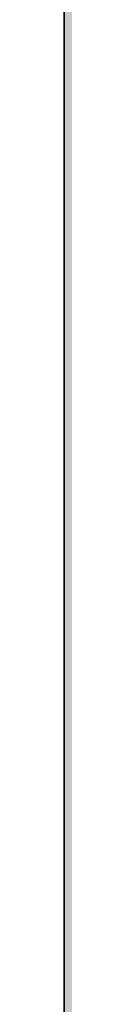
# Model space of a CAD drawing. Units: inches. Extents: x 2091 to 2899, y 967 to 2217.
# Tile 49 of 256: x 2203.14 to 2203.14, y 1096.47 to 1113.86. Entities that reach past the tile are written whole.
import ezdxf

# ---------------------------------------------------------------- set-up
doc = ezdxf.new("R2010")
doc.units = ezdxf.units.IN
doc.layers.add('A-WALL-PATT', color=141, linetype='Continuous', lineweight=13, true_color=0xadddf7)
doc.layers.add('C-PROP', color=7, linetype='Continuous', lineweight=35)

msp = doc.modelspace()

# ---------------------------------------------------------------- hatches: boundary and pattern name
at = {"layer": 'A-WALL-PATT'}
h = msp.add_hatch(color=256, dxfattribs=at)
h.dxf.hatch_style = 1
h.paths.add_polyline_path([(2212.144, 1941.419), (2387.644, 1941.419), (2387.644, 1824.419), (2392.144, 1824.419), (2392.144, 1941.419), (2609.644, 1941.419), (2609.644, 1825.919), (2614.144, 1825.919), (2614.144, 1941.419), (2794.144, 1941.419), (2794.144, 1928.762), (2803.144, 1928.762), (2803.144, 2050.919), (2203.144, 2050.919), (2203.144, 1900.758), (2212.144, 1900.758)])
h.paths.add_polyline_path([(2212.144, 1945.919), (2212.144, 2041.919), (2794.144, 2041.919), (2794.144, 1945.919), (2402.248, 1945.919), (2401.102, 1945.776), (2398.702, 1945.776)], flags=16)
h.paths.add_polyline_path([(2230.23, 1948.063), (2227.35, 1949.503), (2225.91, 1951.903), (2223.99, 1952.863), (2223.03, 1955.263), (2222.07, 1959.583), (2222.07, 1963.423), (2223.03, 1965.663), (2223.99, 1965.343), (2225.586, 1963.861), (2226.912, 1964.957), (2226.949, 1965.939), (2227.778, 1966.952), (2228.2, 1968.879), (2230.71, 1964.863), (2233.59, 1966.303), (2233.607, 1966.332), (2233.773, 1964.938), (2234.634, 1963.676), (2235.03, 1963.903), (2236.282, 1965.572), (2235.99, 1962.943), (2237.955, 1957.54), (2238.39, 1957.903), (2239.216, 1960.306), (2238.655, 1966.385), (2238.693, 1966.438), (2238.841, 1967.5), (2238.78, 1967.687), (2238.881, 1967.787), (2238.667, 1966.252), (2239.216, 1960.306), (2238.39, 1957.903), (2236.95, 1956.703), (2234.55, 1949.983)], flags=0)
h.paths.add_polyline_path([(2278.012, 1948.063), (2276.496, 1947.873), (2275.85, 1947.689), (2274.652, 1947.103)], flags=0)
h.paths.add_polyline_path([(2269.852, 1955.743), (2268.276, 1956.629), (2270.867, 1956.348), (2269.372, 1958.143), (2268.715, 1959.192), (2270.57, 1958.729), (2268.581, 1961.906), (2270.812, 1960.892), (2270.812, 1963.423), (2271.393, 1964.779), (2270.292, 1966.156), (2271.772, 1965.663), (2272.141, 1966.525), (2273.93, 1965.929), (2275.63, 1968.054), (2276.332, 1966.722), (2276.52, 1966.952), (2276.942, 1968.879), (2277.734, 1967.611), (2278.14, 1969.465), (2279.659, 1967.034), (2280.412, 1966.783), (2280.949, 1967.589), (2281.61, 1967.369), (2282.133, 1968.154), (2282.349, 1966.333), (2282.35, 1966.333), (2283.408, 1968.095), (2283.713, 1965.524), (2284.32, 1964.634), (2284.512, 1964.889), (2284.235, 1965.705), (2284.5, 1967.319), (2284.908, 1965.417), (2285.396, 1966.069), (2285.433, 1966.291), (2285.473, 1966.171), (2286.354, 1967.345), (2286.222, 1966.158), (2287.663, 1968.08), (2287.714, 1968.443), (2288.482, 1969.017), (2288.574, 1968.729), (2288.917, 1969.069), (2288.607, 1966.838), (2288.929, 1963.351), (2288.935, 1963.357), (2288.93, 1963.34), (2289.015, 1962.414), (2290.111, 1963.875), (2290.133, 1963.943), (2290.218, 1964.017), (2290.111, 1963.875), (2289.156, 1960.892), (2288.594, 1959.257), (2288.572, 1959.103), (2289.532, 1960.543), (2290.012, 1962.463), (2290.192, 1962.643), (2289.77, 1959.689), (2286.89, 1957.289), (2284.49, 1950.569), (2283.315, 1950.046), (2283.292, 1949.983), (2280.29, 1948.649), (2281.13, 1948.649), (2282.57, 1948.169), (2283.205, 1948.063), (2278.972, 1948.063), (2276.092, 1949.503), (2274.652, 1951.903), (2272.732, 1952.863)], flags=0)
h.paths.add_polyline_path([(2271.159, 1958.022), (2272.97, 1955.849), (2272.01, 1960.169), (2272.01, 1964.009), (2272.624, 1965.443), (2274.328, 1963.861), (2275.654, 1964.957), (2275.638, 1964.539), (2277.412, 1966.007), (2277.033, 1965.157), (2276.83, 1964.976), (2276.766, 1963.295), (2277.45, 1962.66), (2279.452, 1964.863), (2282.332, 1966.303), (2283.53, 1966.889), (2283.295, 1966.771), (2283.913, 1963.885), (2284.899, 1964.448), (2284.732, 1962.943), (2286.697, 1957.54), (2287.132, 1957.903), (2287.542, 1959.095), (2287.779, 1958.442), (2285.683, 1956.695), (2285.877, 1959.795), (2284.732, 1962.943), (2284.899, 1964.448), (2283.913, 1963.885), (2284.224, 1962.434), (2283.424, 1963.605), (2281.61, 1962.569), (2281.13, 1960.169), (2282.09, 1956.329), (2283.05, 1952.969), (2282.57, 1950.569), (2280.17, 1948.649), (2279.883, 1948.792), (2278.972, 1948.063), (2278.972, 1949.023), (2278.672, 1949.397), (2277.29, 1950.089), (2275.85, 1952.489), (2273.93, 1953.449), (2272.49, 1954.889), (2271.922, 1954.889), (2271.772, 1955.263)], flags=0)
h.paths.add_polyline_path([(2311.994, 1955.743), (2312.063, 1955.674), (2312.055, 1955.709)], flags=0)
h.paths.add_polyline_path([(2331.956, 1963.952), (2333.396, 1965.392), (2331.077, 1963.357), (2330.999, 1963.112)], flags=0)
h.paths.add_polyline_path([(2310.554, 1954.303), (2307.04, 1956.28), (2310.763, 1955.876), (2312.474, 1953.823), (2313.434, 1951.423), (2315.354, 1950.463), (2316.794, 1948.063), (2317.466, 1947.727), (2319.369, 1947.965), (2317.754, 1949.983), (2317.57, 1950.61), (2316.794, 1951.903), (2314.874, 1952.863), (2313.914, 1955.263), (2311.514, 1958.143), (2309.375, 1961.559), (2311.514, 1960.337), (2311.514, 1961.983), (2310.605, 1963.12), (2311.727, 1962.479), (2312.418, 1964.093), (2312.256, 1964.296), (2313.194, 1963.983), (2313.914, 1965.663), (2314.647, 1965.419), (2315.354, 1966.303), (2316.794, 1967.743), (2316.157, 1966.947), (2317.034, 1965.282), (2317.223, 1965.512), (2317.777, 1968.046), (2318.474, 1966.722), (2318.663, 1966.952), (2319.084, 1968.879), (2321.207, 1965.482), (2322.161, 1966.914), (2322.554, 1966.783), (2322.786, 1967.131), (2322.882, 1966.324), (2323.312, 1965.722), (2323.651, 1965.891), (2324.396, 1967.133), (2324.657, 1964.938), (2324.972, 1964.477), (2325.387, 1967.001), (2325.941, 1964.418), (2327.229, 1966.136), (2327.166, 1965.572), (2328.059, 1966.763), (2328.225, 1966.247), (2329.668, 1967.677), (2329.665, 1967.687), (2329.765, 1967.787), (2329.551, 1966.252), (2330.1, 1960.306), (2329.333, 1958.073), (2329.313, 1957.935), (2329.634, 1958.203), (2330.234, 1959.103), (2330.714, 1961.023), (2331.034, 1961.343), (2330.714, 1959.103), (2329.634, 1958.203), (2329.274, 1957.663), (2327.712, 1956.361), (2325.434, 1949.983), (2324.334, 1949.494), (2323.994, 1948.543), (2319.674, 1946.623), (2316.794, 1948.063), (2315.354, 1950.463), (2313.434, 1951.423)], flags=0)
h.paths.add_polyline_path([(2321.336, 1947.952), (2321.114, 1948.063), (2321.114, 1949.023), (2319.194, 1951.423), (2316.794, 1959.583), (2316.663, 1959.583), (2315.354, 1958.143), (2314.394, 1958.143), (2313.148, 1958.709), (2312.954, 1959.583), (2312.954, 1960.892), (2315.834, 1959.583), (2316.663, 1959.583), (2317.315, 1960.299), (2315.03, 1962.421), (2316.356, 1963.517), (2316.372, 1963.952), (2316.47, 1963.861), (2317.796, 1964.957), (2317.755, 1963.89), (2319.175, 1965.157), (2319.498, 1965.881), (2321.114, 1965.343), (2323.236, 1962.372), (2325.686, 1963.773), (2325.543, 1962.481), (2325.199, 1963.494), (2324.479, 1963.082), (2324.926, 1960.994), (2324.078, 1962.236), (2322.415, 1961.286), (2322.074, 1959.583), (2323.034, 1955.743), (2323.994, 1952.383), (2323.514, 1949.983), (2322.143, 1948.886), (2322.074, 1948.543)], flags=0)
h.paths.add_polyline_path([(2320.207, 1963.337), (2320.154, 1963.423), (2320.394, 1963.543)], flags=0)
h.paths.add_polyline_path([(2353.851, 1965.811), (2354.031, 1965.751), (2354.331, 1966.451), (2354.331, 1966.931)], flags=0)
h.paths.add_polyline_path([(2359.021, 1969.026), (2359.098, 1968.902), (2359.234, 1969.52), (2359.234, 1970)], flags=0)
h.paths.add_polyline_path([(2358.257, 1966.682), (2357.984, 1966.348), (2358.211, 1966.146), (2358.41, 1966.39)], flags=0)
h.paths.add_polyline_path([(2357.768, 1966.059), (2357.732, 1965.105), (2357.751, 1965.121), (2357.77, 1965.607), (2357.77, 1966.058)], flags=0)
h.paths.add_polyline_path([(2359.112, 1965.305), (2359.112, 1964.825), (2359.845, 1966.468), (2359.845, 1966.948)], flags=0)
h.paths.add_polyline_path([(2360.224, 1966.621), (2360.699, 1969.363), (2360.699, 1969.843), (2360.211, 1967.026), (2360.211, 1966.643)], flags=0)
h.paths.add_polyline_path([(2363.451, 1967.891), (2363.451, 1968.371), (2362.491, 1966.931), (2362.656, 1966.699)], flags=0)
h.paths.add_polyline_path([(2364.476, 1966.079), (2365.851, 1968.371), (2365.851, 1968.851), (2364.428, 1966.48)], flags=0)
h.paths.add_polyline_path([(2366.314, 1965.853), (2366.367, 1965.696), (2366.803, 1968.346), (2366.803, 1968.826)], flags=0)
h.paths.add_polyline_path([(2367.165, 1965.804), (2367.291, 1966.931), (2367.291, 1967.411), (2367.103, 1965.72)], flags=0)
h.paths.add_polyline_path([(2370.037, 1959.974), (2371.014, 1963.025), (2371.014, 1963.505), (2370.037, 1960.454)], flags=0)
h.paths.add_polyline_path([(2371.611, 1960.211), (2372.571, 1961.651), (2372.571, 1962.131), (2371.803, 1960.979)], flags=0)
h.paths.add_polyline_path([(2350.874, 1956.005), (2351.931, 1955.891), (2354.491, 1953.331), (2353.851, 1954.931), (2351.451, 1957.811), (2347.936, 1963.426), (2347.936, 1963.906), (2351.451, 1958.291), (2353.705, 1955.585), (2352.891, 1959.251), (2352.891, 1959.731), (2352.891, 1961.925), (2356.731, 1959.731), (2358.454, 1961.627), (2354.811, 1965.011), (2355.031, 1965.286), (2358.691, 1961.887), (2361.531, 1965.011), (2364.376, 1966.433), (2364.524, 1965.187), (2365.454, 1963.824), (2365.881, 1964.068), (2365.371, 1966.451), (2365.371, 1966.931), (2366.811, 1960.211), (2366.811, 1959.731), (2366.389, 1952.981), (2367.771, 1956.851), (2368.641, 1957.576), (2366.811, 1962.611), (2366.811, 1963.091), (2368.775, 1957.688), (2369.211, 1958.051), (2370.002, 1960.352), (2369.475, 1966.053), (2369.513, 1966.106), (2369.514, 1966.111), (2369.475, 1966.533), (2369.513, 1966.586), (2369.615, 1967.313), (2369.183, 1968.659), (2369.183, 1969.139), (2369.601, 1967.835), (2369.701, 1967.934), (2369.718, 1968.055), (2370.145, 1968.374), (2369.779, 1968.011), (2369.701, 1967.454), (2370.468, 1968.214), (2369.675, 1967.266), (2369.514, 1966.111), (2370.037, 1960.454), (2370.037, 1959.974), (2369.442, 1958.243), (2370.651, 1959.251), (2371.046, 1962.018), (2371.131, 1962.131), (2370.651, 1958.771), (2367.771, 1956.371), (2365.371, 1949.651), (2362.079, 1948.188), (2363.451, 1947.731), (2361.051, 1947.731), (2360.091, 1947.731), (2357.104, 1947.357), (2360.091, 1948.211), (2358.171, 1949.171), (2356.731, 1951.571), (2354.811, 1952.531), (2351.931, 1955.411)], flags=0)
h.paths.add_polyline_path([(2361.051, 1948.691), (2359.131, 1951.091), (2356.731, 1959.251), (2355.771, 1959.251), (2352.891, 1960.56), (2352.891, 1961.445), (2355.891, 1959.731), (2356.731, 1959.731), (2356.837, 1959.368), (2361.531, 1964.531), (2363.248, 1965.389), (2364.925, 1963.042), (2362.491, 1961.651), (2362.064, 1959.517), (2362.971, 1955.891), (2363.931, 1952.531), (2363.931, 1952.051), (2363.451, 1949.651), (2361.051, 1947.731)], flags=0)
h.paths.add_polyline_path([(2359.131, 1951.571), (2359.291, 1951.371), (2361.051, 1954.451), (2361.051, 1954.931)], flags=0)
h.paths.add_polyline_path([(2357.22, 1966.546), (2356.793, 1968.815), (2356.793, 1969.295), (2357.22, 1967.026)], flags=0)
h.paths.add_polyline_path([(2361.051, 1954.451), (2361.531, 1958.771), (2361.531, 1959.251), (2361.051, 1954.931)], flags=0)
h.paths.add_polyline_path([(2402.548, 1948.486), (2402.302, 1948.416), (2402.59, 1948.416)], flags=0)
h.paths.add_polyline_path([(2394.142, 1956.096), (2395.685, 1954.553), (2396.72, 1953.971), (2396.062, 1955.616), (2395.241, 1956.601), (2395.879, 1956.442), (2395.102, 1959.936), (2395.102, 1963.776), (2396.062, 1966.016), (2397.022, 1965.696), (2398.618, 1964.214), (2399.944, 1965.31), (2399.981, 1966.292), (2400.811, 1967.305), (2401.232, 1969.232), (2403.538, 1965.543), (2403.942, 1967.389), (2404.702, 1967.136), (2405.46, 1966.075), (2406.622, 1966.656), (2406.64, 1966.685), (2406.805, 1965.291), (2406.926, 1965.115), (2407.342, 1964.976), (2407.874, 1965.774), (2408.169, 1964.398), (2409.315, 1965.925), (2409.217, 1965.051), (2409.445, 1963.131), (2410.306, 1961.87), (2410.702, 1962.096), (2411.442, 1963.082), (2411.165, 1963.898), (2411.616, 1966.64), (2411.725, 1966.791), (2411.873, 1967.853), (2411.813, 1968.041), (2411.913, 1968.14), (2411.699, 1966.605), (2412.248, 1960.659), (2413.225, 1963.71), (2414.378, 1964.721), (2414.513, 1965.693), (2414.453, 1965.881), (2414.553, 1965.98), (2414.378, 1964.721), (2414.52, 1964.846), (2414.365, 1964.631), (2414.339, 1964.445), (2414.888, 1958.499), (2414.062, 1956.096), (2412.622, 1954.896), (2410.171, 1948.033), (2410.017, 1948.084), (2405.902, 1946.256), (2405.902, 1947.216), (2405.204, 1948.089), (2404.222, 1948.416), (2403.262, 1948.416), (2400.382, 1949.856), (2399.662, 1951.056), (2397.982, 1952.736), (2397.022, 1953.216), (2395.685, 1954.553), (2392.657, 1956.257)], flags=0)
h.paths.add_polyline_path([(2409.086, 1964.407), (2409.13, 1964.276), (2409.262, 1964.496)], flags=0)
h.paths.add_polyline_path([(2397.742, 1961.616), (2398.702, 1963.856), (2399.662, 1963.536), (2401.427, 1965.741), (2401.791, 1966.559), (2402.071, 1965.071), (2402.836, 1964.393), (2403.262, 1964.915), (2403.338, 1964.771), (2402.616, 1963.976), (2402.499, 1960.902), (2403.543, 1959.932), (2404.413, 1960.89), (2404.702, 1962.336), (2407.916, 1964.172), (2409.52, 1961.927), (2410.987, 1957.893), (2411.422, 1958.256), (2412.048, 1960.076), (2412.41, 1959.079), (2411.676, 1958.467), (2411.662, 1958.256), (2411.626, 1958.426), (2409.982, 1957.056), (2407.582, 1950.336), (2403.262, 1948.416), (2403.262, 1949.376), (2401.342, 1951.776), (2399.417, 1958.324), (2397.742, 1959.085), (2397.742, 1959.97), (2397.102, 1960.336), (2397.742, 1960.045)], flags=0)
h.paths.add_polyline_path([(2405.902, 1952.976), (2405.95, 1953.408), (2406.017, 1953.176)], flags=0)
h.paths.add_polyline_path([(2449.818, 1967.114), (2449.752, 1967.136), (2449.794, 1967.078)], flags=0)
h.paths.add_polyline_path([(2451.698, 1966.618), (2451.741, 1966.69), (2451.692, 1966.666)], flags=0)
h.paths.add_polyline_path([(2454.344, 1965.738), (2455.752, 1967.616), (2455.992, 1968.096), (2454.364, 1965.925)], flags=0)
h.paths.add_polyline_path([(2457.547, 1968.864), (2457.787, 1969.344), (2457.054, 1968.796), (2457.008, 1968.46)], flags=0)
h.paths.add_polyline_path([(2456.922, 1967.857), (2456.802, 1968.229), (2456.723, 1967.66)], flags=0)
h.paths.add_polyline_path([(2457.302, 1967.377), (2457.542, 1967.857), (2456.81, 1966.84), (2456.741, 1966.7), (2456.749, 1966.608)], flags=0)
h.paths.add_polyline_path([(2458.275, 1963.71), (2458.155, 1963.335), (2460.354, 1965.265), (2460.594, 1965.745)], flags=0)
h.paths.add_polyline_path([(2458.392, 1962.816), (2458.364, 1962.618), (2459.592, 1964.256), (2459.832, 1964.736)], flags=0)
h.paths.add_polyline_path([(2459.352, 1962.816), (2459.272, 1962.496), (2460.072, 1963.296), (2460.312, 1963.776)], flags=0)
h.paths.add_polyline_path([(2458.68, 1960.608), (2458.632, 1960.416), (2459.592, 1961.856), (2459.832, 1962.336)], flags=0)
h.paths.add_polyline_path([(2437.838, 1956.243), (2439.192, 1956.096), (2441.352, 1953.936), (2440.872, 1955.136), (2438.472, 1958.016), (2438.072, 1958.656), (2438.712, 1958.496), (2440.64, 1956.183), (2439.912, 1959.456), (2439.912, 1963.296), (2441.352, 1966.656), (2441.592, 1967.136), (2441.112, 1966.016), (2442.072, 1965.696), (2443.989, 1968.092), (2444.241, 1966.751), (2444.917, 1966.152), (2445.677, 1967.08), (2446.255, 1969.725), (2446.495, 1970.205), (2446.282, 1969.232), (2447.363, 1967.503), (2447.72, 1969.568), (2447.96, 1970.048), (2447.485, 1967.307), (2448.792, 1965.216), (2448.472, 1964.864), (2448.552, 1964.736), (2451.452, 1966.186), (2451.615, 1964.811), (2452.308, 1963.796), (2453.235, 1964.326), (2454.072, 1960.416), (2453.629, 1953.318), (2454.792, 1956.576), (2455.032, 1957.056), (2455.719, 1957.628), (2453.832, 1962.816), (2453.941, 1963.794), (2453.335, 1965.578), (2453.824, 1968.551), (2454.064, 1969.031), (2453.575, 1966.058), (2454.04, 1964.688), (2453.832, 1962.816), (2455.719, 1957.628), (2456.367, 1958.168), (2457.058, 1960.179), (2457.298, 1960.659), (2456.472, 1958.256), (2457.718, 1959.294), (2457.672, 1958.976), (2454.89, 1956.657), (2453.614, 1953.085), (2453.592, 1952.736), (2453.352, 1952.256), (2453.36, 1952.372), (2452.632, 1950.336), (2452.392, 1949.856), (2449.204, 1948.439), (2450.712, 1947.936), (2448.072, 1947.936), (2447.112, 1947.936), (2444.552, 1947.616), (2447.2, 1948.372), (2445.192, 1949.376), (2443.752, 1951.776), (2441.832, 1952.736), (2438.952, 1955.616)], flags=0)
h.paths.add_polyline_path([(2443.992, 1959.936), (2444.04, 1959.773), (2444.122, 1959.862)], flags=0)
h.paths.add_polyline_path([(2442.912, 1959.936), (2443.032, 1959.936), (2442.446, 1960.202)], flags=0)
h.paths.add_polyline_path([(2444.983, 1965.02), (2445.279, 1965.265), (2445.519, 1965.745), (2444.994, 1965.31)], flags=0)
h.paths.add_polyline_path([(2446.133, 1965.03), (2446.33, 1965.471), (2444.97, 1964.258), (2444.73, 1963.778)], flags=0)
h.paths.add_polyline_path([(2442.792, 1959.456), (2443.752, 1959.456), (2446.152, 1951.296), (2446.412, 1951.751), (2446.392, 1951.776), (2448.081, 1954.73), (2448.552, 1958.976), (2441.832, 1965.216), (2442.155, 1965.619), (2448.792, 1959.456), (2448.312, 1955.136), (2448.072, 1954.656), (2446.412, 1951.751), (2448.312, 1949.376), (2448.312, 1948.416), (2450.541, 1950.199), (2450.952, 1952.256), (2449.992, 1955.616), (2449.032, 1959.456), (2449.512, 1961.856), (2449.752, 1962.336), (2449.675, 1961.949), (2452.995, 1963.846), (2453.064, 1963.519), (2452.885, 1963.783), (2449.675, 1961.949), (2449.272, 1959.936), (2450.232, 1956.096), (2451.192, 1952.736), (2450.712, 1950.336), (2450.472, 1949.856), (2448.072, 1947.936), (2448.072, 1948.536), (2445.432, 1949.856), (2443.992, 1952.256), (2442.072, 1953.216), (2441.112, 1955.616), (2440.152, 1959.936), (2440.152, 1960.656)], flags=0)
h.paths.add_polyline_path([(2456.692, 1966.986), (2457.608, 1968.081), (2457.848, 1968.561), (2456.932, 1967.466)], flags=0)
h.paths.add_polyline_path([(2489.897, 1966.58), (2489.943, 1966.189), (2490.747, 1967.53), (2491.319, 1968.951)], flags=0)
h.paths.add_polyline_path([(2473.562, 1956.407), (2477.14, 1956.019), (2476.955, 1956.241), (2475.108, 1957.28), (2476.347, 1956.97), (2475.187, 1958.824), (2476.919, 1958.391), (2475.412, 1960.799), (2477.787, 1959.719), (2477.787, 1962.25), (2477.637, 1962.438), (2477.823, 1962.332), (2478.359, 1963.584), (2478.359, 1963.671), (2477.324, 1964.965), (2478.715, 1964.501), (2479.319, 1965.911), (2480.279, 1965.591), (2481.784, 1967.472), (2482.116, 1965.705), (2482.881, 1965.028), (2483.209, 1965.429), (2483.22, 1965.715), (2483.076, 1965.989), (2483.712, 1966.766), (2484.13, 1968.679), (2484.702, 1970.1), (2484.489, 1969.127), (2486.503, 1965.905), (2487.387, 1965.61), (2488.153, 1966.759), (2488.717, 1965.97), (2489.2, 1966.212), (2489.331, 1965.111), (2490.394, 1963.622), (2490.661, 1963.775), (2490.494, 1964.554), (2490.923, 1963.925), (2491.319, 1964.151), (2491.333, 1964.17), (2491.21, 1964.532), (2491.282, 1964.966), (2491.426, 1964.293), (2494.076, 1967.828), (2494.498, 1966.515), (2494.598, 1966.614), (2494.689, 1967.27), (2495.107, 1967.582), (2495.13, 1967.748), (2495.07, 1967.936), (2495.17, 1968.035), (2495.032, 1967.044), (2495.754, 1967.759), (2494.982, 1966.686), (2494.956, 1966.5), (2495.479, 1960.837), (2495.91, 1962.184), (2496.482, 1963.605), (2496.073, 1962.327), (2496.769, 1962.938), (2496.599, 1962.711), (2496.119, 1959.351), (2496.733, 1960.272), (2496.987, 1961.29), (2497.559, 1962.711), (2497.079, 1960.791), (2496.507, 1959.37), (2495.547, 1957.93), (2492.759, 1955.606), (2490.839, 1950.231), (2490.267, 1948.81), (2485.947, 1946.89), (2483.067, 1948.33), (2481.627, 1950.73), (2479.707, 1951.69), (2476.827, 1954.57)], flags=0)
h.paths.add_polyline_path([(2485.577, 1948.313), (2485.559, 1948.311), (2485.579, 1948.311)], flags=0)
h.paths.add_polyline_path([(2478.645, 1954.551), (2478.109, 1956.963), (2479.319, 1955.511), (2480.279, 1953.111), (2482.199, 1952.151), (2483.639, 1949.751), (2486.519, 1948.311), (2486.519, 1949.271), (2484.739, 1951.496), (2484.027, 1950.25), (2481.627, 1958.41), (2482.375, 1959.233), (2482.199, 1959.831), (2483.198, 1960.929), (2479.707, 1964.17), (2480.603, 1965.29), (2481.875, 1964.109), (2482.666, 1964.764), (2482.615, 1963.422), (2482.989, 1963.075), (2484.008, 1963.984), (2484.684, 1965.498), (2484.58, 1965.405), (2485.357, 1967.147), (2485.121, 1965.781), (2486.427, 1963.69), (2488.145, 1964.549), (2489.822, 1962.202), (2490.747, 1962.73), (2492, 1964.4), (2492.076, 1965.087), (2492.213, 1964.684), (2492.485, 1965.047), (2492.279, 1963.191), (2494.244, 1957.788), (2494.563, 1958.054), (2494.933, 1959.133), (2495.505, 1960.554), (2494.679, 1958.151), (2494.107, 1956.73), (2494.563, 1958.054), (2493.409, 1957.092), (2491.707, 1961.77), (2492, 1964.4), (2490.747, 1962.73), (2487.712, 1960.996), (2487.479, 1959.831), (2488.439, 1955.991), (2489.399, 1952.631), (2488.919, 1950.231), (2488.577, 1949.957), (2488.347, 1948.81), (2487.652, 1948.254), (2487.479, 1948.311), (2486.519, 1948.311), (2483.639, 1949.751), (2482.199, 1952.151), (2480.279, 1953.111), (2478.839, 1954.551)], flags=0)
h.paths.add_polyline_path([(2526.648, 1966.988), (2526.517, 1967.031), (2526.6, 1966.915)], flags=0)
h.paths.add_polyline_path([(2528.471, 1966.447), (2528.574, 1966.62), (2528.457, 1966.561)], flags=0)
h.paths.add_polyline_path([(2534.133, 1967.496), (2534.157, 1967.543), (2534.06, 1967.408)], flags=0)
h.paths.add_polyline_path([(2536.162, 1964.051), (2535.157, 1962.711), (2535.101, 1962.316), (2536.117, 1963.671), (2536.421, 1964.278)], flags=0)
h.paths.add_polyline_path([(2535.157, 1959.831), (2536.117, 1961.271), (2536.597, 1962.231), (2535.253, 1960.215)], flags=0)
h.paths.add_polyline_path([(2513.249, 1956.285), (2516.221, 1955.963), (2514.997, 1957.431), (2514.196, 1958.712), (2515.477, 1958.391), (2516.932, 1956.646), (2516.437, 1958.871), (2516.437, 1962.711), (2516.873, 1963.727), (2515.346, 1965.635), (2517.397, 1964.951), (2517.877, 1966.071), (2518.357, 1967.031), (2517.877, 1965.911), (2518.837, 1965.591), (2520.487, 1967.653), (2520.766, 1966.166), (2521.53, 1965.489), (2521.781, 1965.795), (2521.801, 1966.307), (2521.478, 1966.921), (2521.246, 1967.126), (2521.178, 1967.491), (2521.478, 1966.921), (2522.01, 1966.449), (2522.257, 1966.75), (2522.78, 1969.14), (2523.26, 1970.1), (2523.047, 1969.127), (2524.673, 1966.526), (2526.037, 1966.071), (2526.795, 1965.01), (2527.977, 1965.601), (2528.14, 1964.227), (2528.665, 1963.458), (2529.389, 1963.872), (2529.33, 1964.147), (2529.481, 1963.925), (2529.877, 1964.151), (2529.984, 1964.293), (2529.789, 1965.203), (2530.062, 1964.398), (2532.802, 1968.051), (2533.148, 1966.976), (2533.248, 1967.075), (2533.339, 1967.731), (2533.673, 1967.98), (2533.728, 1968.035), (2533.514, 1966.5), (2534.025, 1960.972), (2534.56, 1962.645), (2535.04, 1963.605), (2534.063, 1960.554), (2533.237, 1958.151), (2534.288, 1959.027), (2534.197, 1958.391), (2531.513, 1956.154), (2529.397, 1950.231), (2528.917, 1949.271), (2526.449, 1948.174), (2527.477, 1947.831), (2530.357, 1947.351), (2524.597, 1947.351), (2521.717, 1948.791), (2520.277, 1951.191), (2518.357, 1952.151), (2515.477, 1955.031)], flags=0)
h.paths.add_polyline_path([(2523.935, 1967.19), (2523.62, 1966.484), (2523.77, 1966.242)], flags=0)
h.paths.add_polyline_path([(2518.837, 1953.111), (2517.877, 1955.511), (2516.885, 1959.977), (2516.917, 1959.962), (2516.917, 1962.025), (2520.757, 1959.831), (2522.025, 1961.226), (2518.357, 1964.631), (2519.003, 1965.438), (2520.433, 1964.109), (2521.301, 1964.827), (2521.245, 1963.355), (2525.638, 1959.276), (2526.037, 1961.271), (2529.397, 1963.191), (2530.65, 1964.861), (2530.665, 1964.998), (2530.692, 1964.917), (2531.088, 1965.445), (2530.946, 1964.169), (2530.692, 1964.917), (2529.397, 1963.191), (2526.363, 1961.457), (2526.037, 1959.831), (2526.997, 1955.991), (2527.957, 1952.631), (2527.477, 1950.231), (2527.134, 1949.957), (2526.974, 1949.154), (2526.697, 1949.031), (2524.597, 1947.351), (2524.597, 1948.311), (2524.277, 1948.711), (2522.197, 1949.751), (2520.757, 1952.151)], flags=0)
h.paths.add_polyline_path([(2520.277, 1958.871), (2520.853, 1959.505), (2523.157, 1951.671), (2524.614, 1954.22), (2524.597, 1954.071), (2522.677, 1950.711)], flags=0)
h.paths.add_polyline_path([(2559.371, 1966.311), (2559.398, 1966.325), (2559.402, 1966.345)], flags=0)
h.paths.add_polyline_path([(2549.771, 1957.191), (2552.651, 1954.311), (2552.134, 1955.603), (2550.611, 1957.431), (2547.096, 1963.046), (2545.776, 1965.206), (2549.291, 1959.591), (2551.691, 1956.711), (2550.793, 1960.752), (2550.731, 1960.78), (2550.731, 1964.871), (2551.691, 1967.111), (2552.651, 1966.791), (2554.247, 1965.309), (2555.034, 1965.96), (2555.582, 1966.645), (2555.61, 1967.387), (2556.439, 1968.401), (2556.861, 1970.327), (2559.371, 1966.311), (2560.691, 1964.151), (2562.409, 1965.01), (2561.651, 1966.071), (2560.331, 1968.231), (2561.758, 1966.233), (2562.347, 1967.116), (2562.434, 1966.387), (2563.128, 1965.37), (2563.571, 1965.591), (2563.588, 1965.62), (2563.363, 1967.524), (2563.722, 1965.844), (2565.06, 1968.073), (2564.733, 1965.129), (2565.118, 1963.333), (2567.445, 1966.436), (2567.316, 1967.833), (2567.354, 1967.886), (2567.502, 1968.948), (2567.441, 1969.136), (2567.542, 1969.235), (2567.328, 1967.7), (2567.877, 1961.754), (2568.747, 1964.47), (2568.636, 1965.673), (2568.674, 1965.726), (2568.822, 1966.788), (2568.761, 1966.976), (2568.862, 1967.075), (2568.648, 1965.54), (2568.726, 1964.693), (2568.854, 1964.805), (2568.747, 1964.47), (2568.817, 1963.706), (2568.971, 1963.911), (2568.866, 1963.177), (2569.197, 1959.594), (2568.371, 1957.191), (2566.931, 1955.991), (2564.62, 1949.521), (2564.651, 1949.511), (2564.617, 1949.511), (2564.531, 1949.271), (2560.211, 1947.351), (2557.331, 1948.791), (2556.045, 1950.934), (2556.011, 1950.951), (2555.857, 1951.208), (2553.971, 1952.151), (2551.091, 1955.031), (2546.65, 1957.53)], flags=0)
h.paths.add_polyline_path([(2567.026, 1959.33), (2567.035, 1959.305), (2567.051, 1959.351)], flags=0)
h.paths.add_polyline_path([(2551.968, 1962.518), (2553.011, 1964.951), (2553.971, 1964.631), (2555.567, 1963.149), (2556.893, 1964.246), (2556.93, 1965.227), (2557.144, 1965.489), (2556.42, 1966.131), (2556.391, 1966.105), (2556.38, 1966.166), (2556.42, 1966.131), (2556.952, 1966.605), (2557.092, 1966.919), (2557.571, 1966.01), (2557.759, 1966.241), (2557.418, 1964.68), (2556.893, 1964.246), (2556.807, 1961.998), (2560.691, 1958.391), (2560.636, 1957.893), (2560.811, 1957.191), (2561.771, 1953.831), (2561.291, 1951.431), (2559.11, 1949.687), (2559.156, 1949.629), (2563.027, 1951.349), (2562.611, 1949.271), (2560.211, 1947.351), (2560.211, 1948.311), (2559.251, 1949.511), (2558.891, 1949.511), (2558.891, 1949.961), (2558.291, 1950.711), (2558.054, 1951.518), (2556.971, 1952.871), (2555.068, 1959.341), (2552.051, 1961.065), (2552.051, 1962.471)], flags=0)
h.paths.add_polyline_path([(2588.33, 1958.391), (2588.61, 1958.111), (2588.553, 1958.367)], flags=0)
h.paths.add_polyline_path([(2594.745, 1950.493), (2593.958, 1953.172), (2593.13, 1954.551), (2591.21, 1955.511), (2590.25, 1957.911), (2588.309, 1960.24), (2586.177, 1961.209), (2587.85, 1960.791), (2587.253, 1961.744), (2588.441, 1961.065), (2588.441, 1962.656), (2588.422, 1962.665), (2588.441, 1962.711), (2586.914, 1964.62), (2588.877, 1963.728), (2589.29, 1964.692), (2589.29, 1966.071), (2590.25, 1968.311), (2591.21, 1967.991), (2592.806, 1966.509), (2594.132, 1967.606), (2594.169, 1968.587), (2594.999, 1969.601), (2595.42, 1971.527), (2597.93, 1967.511), (2600.81, 1968.951), (2600.827, 1968.98), (2600.993, 1967.587), (2601.854, 1966.325), (2602.107, 1966.47), (2602.236, 1967.255), (2602.357, 1966.693), (2603.502, 1968.221), (2603.21, 1965.591), (2605.175, 1960.188), (2605.507, 1960.465), (2605.026, 1965.673), (2605.064, 1965.726), (2605.212, 1966.788), (2605.152, 1966.976), (2605.252, 1967.075), (2605.343, 1967.731), (2605.953, 1968.187), (2605.875, 1969.033), (2605.913, 1969.086), (2606.061, 1970.148), (2606, 1970.336), (2606.101, 1970.435), (2605.887, 1968.9), (2606.436, 1962.954), (2605.61, 1960.551), (2605.997, 1960.874), (2606.564, 1962.645), (2608.241, 1964.117), (2608.01, 1963.191), (2607.05, 1961.751), (2606.631, 1961.402), (2606.201, 1958.391), (2603.321, 1955.991), (2600.921, 1949.271), (2596.601, 1947.351), (2593.721, 1948.791), (2592.857, 1950.231), (2592.65, 1950.231)], flags=0)
h.paths.add_polyline_path([(2596.601, 1947.351), (2596.601, 1948.311), (2594.681, 1950.711), (2596.155, 1953.29), (2595.53, 1954.071), (2593.199, 1961.996), (2592.651, 1962.505), (2591.78, 1963.003), (2593.283, 1964.246), (2593.32, 1965.227), (2594.15, 1966.241), (2594.571, 1968.167), (2596.183, 1965.589), (2596.951, 1966.435), (2598.041, 1966.071), (2598.799, 1965.01), (2599.961, 1965.591), (2599.979, 1965.62), (2600.144, 1964.227), (2601.005, 1962.965), (2601.401, 1963.191), (2602.653, 1964.861), (2602.361, 1962.231), (2603.793, 1958.295), (2601.978, 1953.212), (2601.946, 1952.709), (2599.469, 1951.608), (2599.001, 1949.271)], flags=0)
h.paths.add_polyline_path([(2597.561, 1958.871), (2597.671, 1959.419), (2597.595, 1958.736)], flags=0)
h.paths.add_polyline_path([(2623.666, 1961.254), (2625.519, 1960.791), (2624.966, 1961.676), (2627.199, 1960.66), (2627.199, 1961.151), (2626.959, 1962.231), (2626.959, 1963.491), (2625.582, 1965.212), (2626.959, 1964.425), (2626.959, 1965.831), (2626.869, 1965.861), (2627.919, 1968.311), (2628.879, 1967.991), (2630.475, 1966.509), (2631.801, 1967.606), (2631.838, 1968.587), (2632.668, 1969.601), (2633.089, 1971.527), (2635.599, 1967.511), (2638.479, 1968.951), (2638.497, 1968.98), (2638.662, 1967.587), (2639.176, 1966.833), (2639.78, 1967.84), (2640.026, 1966.693), (2641.171, 1968.221), (2640.879, 1965.591), (2641.114, 1964.945), (2641.411, 1965.341), (2641.308, 1964.412), (2642.844, 1960.188), (2643.279, 1960.551), (2644.085, 1962.895), (2643.784, 1966.153), (2643.807, 1966.185), (2643.601, 1968.418), (2643.523, 1968.661), (2643.73, 1970.148), (2643.67, 1970.336), (2643.77, 1970.435), (2643.556, 1968.9), (2643.601, 1968.418), (2643.91, 1967.456), (2644.01, 1967.555), (2643.812, 1966.132), (2644.105, 1962.954), (2644.239, 1961.351), (2644.719, 1961.751), (2645.033, 1962.222), (2645.322, 1963.125), (2646.076, 1963.787), (2645.033, 1962.222), (2644.345, 1960.074), (2643.519, 1957.671), (2642.079, 1956.471), (2639.72, 1949.864), (2639.876, 1949.838), (2635.359, 1947.831), (2632.479, 1949.271), (2631.039, 1951.671), (2629.119, 1952.631), (2628.159, 1955.031), (2625.759, 1957.911)], flags=0)
h.paths.add_polyline_path([(2627.816, 1956.574), (2627.374, 1958.566), (2626.376, 1959.763), (2627.199, 1959.351), (2627.374, 1958.566), (2627.919, 1957.911), (2628.879, 1955.511), (2630.799, 1954.551), (2632.239, 1952.151), (2633.315, 1951.613), (2631.039, 1959.351), (2631.498, 1959.856), (2630.799, 1962.231), (2631.45, 1962.947), (2630.715, 1963.629), (2632.041, 1964.726), (2632.078, 1965.707), (2632.292, 1965.969), (2631.705, 1966.489), (2633.136, 1967.766), (2633.329, 1968.647), (2634.675, 1966.494), (2635.208, 1967.081), (2636.799, 1966.551), (2637.676, 1967.867), (2638.994, 1966.022), (2639.705, 1966.429), (2641.119, 1959.831), (2640.93, 1956.806), (2639.439, 1952.631), (2638.227, 1952.093), (2637.759, 1949.751), (2635.359, 1947.831), (2635.359, 1948.791), (2633.439, 1951.191), (2633.315, 1951.613), (2632.239, 1952.151), (2630.799, 1954.551), (2628.879, 1955.511)], flags=0)
h.paths.add_polyline_path([(2637.759, 1953.831), (2637.279, 1955.511), (2636.319, 1959.351), (2636.799, 1961.751), (2639.234, 1963.142), (2637.557, 1965.49), (2638.739, 1966.081), (2638.902, 1964.707), (2639.763, 1963.445), (2636.799, 1961.751), (2636.532, 1960.418), (2637.039, 1958.391), (2637.999, 1955.031)], flags=0)
h.paths.add_polyline_path([(2668.567, 1951.431), (2667.607, 1953.831), (2665.207, 1956.711), (2662.294, 1961.365), (2665.447, 1959.591), (2666.647, 1958.391), (2666.647, 1959.975), (2666.058, 1960.682), (2666.647, 1960.345), (2666.647, 1961.991), (2666.7, 1962.114), (2666.407, 1963.431), (2666.407, 1967.271), (2667.367, 1969.511), (2668.327, 1969.191), (2669.923, 1967.709), (2671.249, 1968.806), (2671.286, 1969.787), (2672.116, 1970.801), (2672.537, 1972.727), (2675.047, 1968.711), (2677.927, 1970.151), (2677.945, 1970.18), (2678.11, 1968.787), (2678.971, 1967.525), (2679.367, 1967.751), (2680.62, 1969.421), (2680.327, 1966.791), (2682.292, 1961.388), (2682.727, 1961.751), (2683.358, 1963.587), (2683.232, 1964.953), (2683.27, 1965.006), (2683.393, 1965.889), (2683.36, 1966.249), (2683.358, 1966.256), (2683.359, 1966.257), (2682.992, 1970.233), (2683.03, 1970.286), (2683.178, 1971.348), (2683.118, 1971.536), (2683.218, 1971.635), (2683.004, 1970.1), (2683.359, 1966.257), (2683.458, 1966.355), (2683.393, 1965.889), (2683.414, 1965.665), (2684.424, 1966.872), (2683.553, 1964.154), (2683.358, 1963.587), (2683.793, 1958.874), (2682.967, 1956.471), (2681.527, 1955.271), (2680.109, 1951.3), (2680.085, 1950.912), (2679.977, 1950.93), (2679.127, 1948.551), (2674.807, 1946.631), (2671.927, 1948.071), (2670.487, 1950.471)], flags=0)
h.paths.add_polyline_path([(2671.936, 1953.227), (2671.687, 1953.351), (2670.247, 1955.751), (2668.327, 1956.711), (2667.357, 1959.138), (2669.527, 1958.151), (2670.487, 1958.151), (2671.479, 1959.242), (2670.684, 1961.945), (2668.89, 1963.612), (2667.307, 1964.331), (2668.567, 1963.911), (2668.831, 1964.241), (2670.247, 1963.431), (2672.422, 1965.823), (2672.777, 1967.447), (2673.234, 1966.716), (2674.412, 1968.012), (2673.981, 1965.522), (2675.287, 1963.431), (2675.554, 1963.564), (2675.932, 1965.456), (2676.247, 1965.351), (2677.005, 1964.29), (2678.167, 1964.871), (2679.607, 1967.271), (2680.327, 1963.911), (2680.307, 1963.577), (2680.347, 1963.458), (2680.86, 1964.141), (2680.567, 1961.511), (2681.104, 1960.037), (2678.887, 1953.831), (2677.092, 1953.033), (2677.687, 1950.951), (2677.207, 1948.551), (2674.807, 1946.631), (2674.807, 1947.591), (2672.887, 1949.991)], flags=0)
h.paths.add_polyline_path([(2673.985, 1951.911), (2674.567, 1952.931), (2674.567, 1951.911), (2676.967, 1953.831), (2677.447, 1956.231), (2676.487, 1959.591), (2676.247, 1960.551), (2679.73, 1962.541), (2680.059, 1961.002), (2679.211, 1962.245), (2676.247, 1960.551), (2676.487, 1959.591), (2677.447, 1956.231), (2676.967, 1953.831), (2674.567, 1951.911)], flags=0)
h.paths.add_polyline_path([(2707.479, 1952.815), (2706.519, 1955.215), (2705.559, 1959.535), (2705.559, 1963.375), (2706.519, 1965.615), (2707.479, 1965.295), (2709.075, 1963.813), (2710.401, 1964.909), (2710.438, 1965.891), (2711.268, 1966.904), (2711.689, 1968.831), (2714.199, 1964.815), (2717.079, 1966.255), (2717.097, 1966.284), (2717.262, 1964.89), (2718.123, 1963.628), (2718.519, 1963.855), (2719.771, 1965.524), (2719.479, 1962.895), (2721.444, 1957.492), (2721.879, 1957.855), (2722.705, 1960.258), (2722.144, 1966.337), (2722.182, 1966.39), (2722.33, 1967.452), (2722.27, 1967.639), (2722.37, 1967.739), (2722.156, 1966.204), (2722.705, 1960.258), (2721.879, 1957.855), (2720.439, 1956.655), (2718.039, 1949.935), (2713.719, 1948.015), (2710.839, 1949.455), (2709.399, 1951.855)], flags=0)
h.paths.add_polyline_path([(2749.301, 1952.815), (2748.341, 1955.215), (2747.381, 1959.535), (2747.381, 1963.375), (2748.341, 1965.615), (2749.301, 1965.295), (2750.897, 1963.813), (2752.223, 1964.909), (2752.26, 1965.891), (2753.09, 1966.904), (2753.511, 1968.831), (2756.021, 1964.815), (2758.901, 1966.255), (2758.919, 1966.284), (2759.084, 1964.89), (2759.945, 1963.628), (2760.341, 1963.855), (2761.593, 1965.524), (2761.301, 1962.895), (2763.266, 1957.492), (2763.701, 1957.855), (2764.527, 1960.258), (2763.966, 1966.337), (2764.004, 1966.39), (2764.152, 1967.452), (2764.092, 1967.639), (2764.192, 1967.739), (2763.978, 1966.204), (2764.527, 1960.258), (2763.701, 1957.855), (2762.261, 1956.655), (2759.861, 1949.935), (2755.541, 1948.015), (2752.661, 1949.455), (2751.221, 1951.855)], flags=0)
h.paths.add_polyline_path([(2212.144, 1819.935), (2203.144, 1819.935), (2203.144, 1739.98), (2212.144, 1739.98), (2212.144, 1780.919), (2392.144, 1780.919), (2392.144, 1783.919), (2212.144, 1783.919)])
h.paths.add_polyline_path([(2803.144, 1847.939), (2794.144, 1847.939), (2794.144, 1785.419), (2609.644, 1785.419), (2493.876, 1785.419), (2493.876, 1780.919), (2609.644, 1780.919), (2794.144, 1780.919), (2794.144, 1696.919), (2609.376, 1696.919), (2609.376, 1742.919), (2604.876, 1742.919), (2604.876, 1644.419), (2609.376, 1644.419), (2609.376, 1692.419), (2794.144, 1692.419), (2794.144, 1668.165), (2803.144, 1668.165)])
h.paths.add_polyline_path([(2392.144, 1740.419), (2387.644, 1740.419), (2387.644, 1629.419), (2212.144, 1629.419), (2212.144, 1659.156), (2203.144, 1659.156), (2203.144, 1494.089), (2212.144, 1494.089), (2212.144, 1627.919), (2392.144, 1627.919)])
h.paths.add_polyline_path([(2457.876, 1780.919), (2453.376, 1780.919), (2453.376, 1644.419), (2568.876, 1644.419), (2568.876, 1648.919), (2457.876, 1648.919)])
h.paths.add_polyline_path([(2545.144, 1591.919), (2540.644, 1591.919), (2540.644, 1567.919), (2468.644, 1567.919), (2468.644, 1627.919), (2509.144, 1627.919), (2509.144, 1632.419), (2464.144, 1632.419), (2464.144, 1563.419), (2545.144, 1563.419)])
h.paths.add_polyline_path([(2268.644, 1555.919), (2212.144, 1555.919), (2212.144, 1551.419), (2268.644, 1551.419)], flags=17)
h.paths.add_polyline_path([(2212.144, 1413.266), (2203.144, 1413.266), (2203.144, 1233.07), (2212.144, 1233.07)])
h.paths.add_polyline_path([(2267.644, 1351.919), (2212.144, 1351.919), (2212.144, 1347.419), (2267.644, 1347.419)], flags=17)
h.paths.add_polyline_path([(2456.644, 1489.419), (2452.144, 1489.419), (2452.144, 1351.919), (2312.644, 1351.919), (2312.644, 1347.419), (2456.644, 1347.419)])
h.paths.add_polyline_path([(2472.37, 1455.419), (2467.87, 1455.419), (2467.87, 1347.419), (2472.37, 1347.419)])
h.paths.add_polyline_path([(2794.144, 1351.919), (2543.37, 1351.919), (2543.37, 1347.419), (2794.144, 1347.419)], flags=17)
h.paths.add_polyline_path([(2312.644, 1347.419), (2308.144, 1347.419), (2308.144, 1302.162), (2308.342, 1302.164), (2308.144, 1298.169), (2308.144, 1275.419), (2212.144, 1275.419), (2212.144, 1270.919), (2312.644, 1270.919)], flags=17)
h.paths.add_polyline_path([(2212.144, 1152.247), (2203.144, 1152.247), (2203.144, 1090.919), (2803.144, 1090.919), (2803.144, 1392.714), (2794.144, 1392.714), (2794.144, 1143.419), (2548.032, 1143.419), (2548.032, 1138.919), (2794.144, 1138.919), (2794.144, 1099.919), (2212.144, 1099.919)])
h.paths.add_polyline_path([(2471.532, 1266.329, 0.031658), (2467.032, 1269.946), (2467.032, 1143.419), (2471.532, 1143.419), (2471.532, 1148.819)], flags=17)
h.paths.add_polyline_path([(2803.144, 1587.341), (2794.144, 1587.341), (2794.144, 1473.537), (2803.144, 1473.537)])
h.paths.add_polyline_path([(2794.144, 1536.419), (2651.144, 1536.419), (2651.144, 1531.919), (2794.144, 1531.919)])
h.paths.add_polyline_path([(2614.144, 1620.419), (2609.644, 1620.419), (2609.644, 1536.419), (2614.144, 1536.419)])
h.paths.add_polyline_path([(2271.083, 1964.317), (2776.853, 1964.317), (2776.853, 2037.17), (2271.083, 2037.17)], flags=8)
h.paths.add_polyline_path([(2380.649, 1536.824), (2461.041, 1536.824), (2461.041, 1554.653), (2380.649, 1554.653)], flags=9)
h.paths.add_polyline_path([(2203.655, 1608.815), (2316.118, 1608.815), (2316.118, 1621.918), (2203.655, 1621.918)], flags=24)
h.paths.add_polyline_path([(2212.677, 1313.504), (2282.592, 1313.504), (2282.592, 1322.745), (2212.677, 1322.745)], flags=24)
h.paths.add_polyline_path([(2457.112, 1114.779), (2558.482, 1114.779), (2558.482, 1142.22), (2457.112, 1142.22)], flags=25)
h.paths.add_polyline_path([(2473.442, 1273.01), (2604.641, 1273.01), (2604.641, 1318.347), (2473.442, 1318.347)], flags=25)
h.paths.add_polyline_path([(2638.876, 1626.977), (2684.25, 1627.977), (2684.038, 1637.597), (2638.664, 1636.598)], flags=9)
h.paths.add_polyline_path([(2537.591, 1453.793), (2628.39, 1453.793), (2628.39, 1475.345), (2537.591, 1475.345)], flags=9)
h.paths.add_polyline_path([(2504.138, 1714.632), (2554.647, 1714.632), (2554.647, 1730.238), (2504.138, 1730.238)], flags=25)
h.paths.add_polyline_path([(2487.501, 1575.652), (2535.097, 1575.652), (2535.097, 1598.378), (2487.501, 1598.378)], flags=25)
h.paths.add_polyline_path([(2709.099, 1735.71), (2740.017, 1735.71), (2740.017, 1749.938), (2709.099, 1749.938)], flags=25)
h.paths.add_polyline_path([(2442.438, 1792.172), (2564.729, 1792.172), (2564.729, 1842), (2442.438, 1842)], flags=9)
h.paths.add_polyline_path([(2655.816, 1809.644), (2789.52, 1806.694), (2790.085, 1832.292), (2656.381, 1835.242)], flags=25)
h.paths.add_polyline_path([(2234.843, 1797.72), (2368.593, 1794.769), (2369.161, 1820.504), (2235.411, 1823.455)], flags=9)
h.paths.add_polyline_path([(2245.138, 1644.006), (2398.428, 1640.624), (2398.995, 1666.325), (2245.706, 1669.707)], flags=9)
h.paths.add_polyline_path([(2306.143, 1431.169), (2413.768, 1428.794), (2414.333, 1454.392), (2306.708, 1456.766)], flags=9)
h.paths.add_polyline_path([(2306.835, 1458.233), (2393.38, 1456.323), (2393.933, 1481.354), (2307.387, 1483.264)], flags=9)

# ---------------------------------------------------------------- linework, layer by layer
at = {"layer": 'C-PROP'}
msp.add_lwpolyline([(2203.144, 2050.919), (2803.144, 2050.919), (2803.144, 1090.919), (2203.144, 1090.919)], close=True, dxfattribs=at)

doc.saveas('drawing.dxf')
